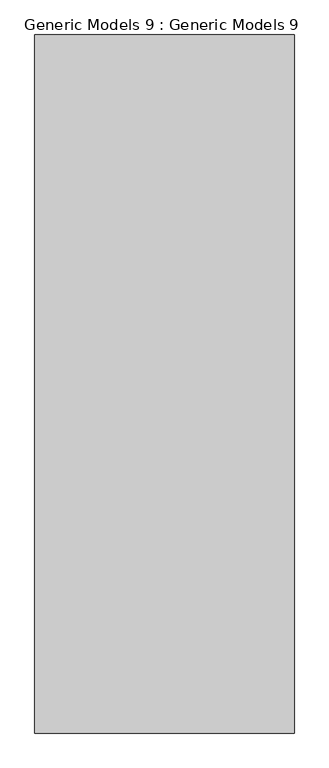
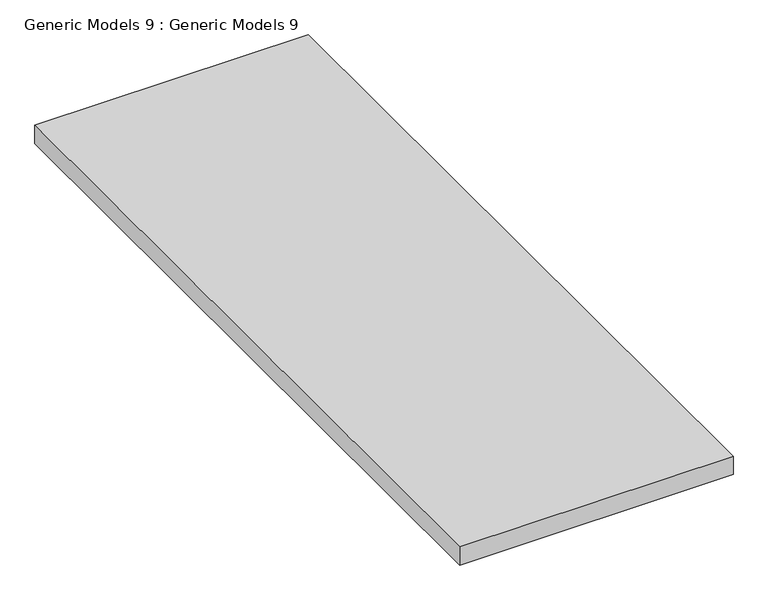
"""IFC4 building model written with IfcOpenShell, lengths in millimetres: proxy geometry, Generic Models 9 : Generic Models 9."""

from ifc_helpers import new_model, si_unit, frame, origin, place, context, project, spatial, polyline, outline, extrude, source, transform, mapped, element, save


def generic_models_9_generic_models_9_5a9dd815(model_context):
    return source(origin(), model_context, "Body", "SweptSolid", [
        extrude(outline(polyline([(-3736.8593778, -7976.2951755), (-5910.1906521, -7976.2951755), (-5910.1906521, -2131.7746485), (-3736.8593778, -2131.7746485), (-3736.8593778, -7976.2951755)])), frame((0.0, 0.0, 7010.4), z_axis=(0.0, 0.0, 1.0), x_axis=(1.0, 0.0, 0.0)), (0.0, 0.0, 1.0), 152.4),
    ])


if __name__ == "__main__":
    model = new_model("IFC4")
    model_context = context("Model", 3, world=origin())
    ifc_project = project(units=[si_unit("LENGTHUNIT", "METRE", prefix="MILLI")], contexts=[model_context])
    site = spatial("IfcSite", under=ifc_project)
    building = spatial("IfcBuilding", under=site)
    placement = place(None, origin())
    generic_models_9_generic_models_9_shape = generic_models_9_generic_models_9_5a9dd815(model_context)
    element("IfcBuildingElementProxy", 1, Name="Generic Models 9 : Generic Models 9", ObjectType="Generic Models 9 : Generic Models 9", at=placement, inside=building, context=model_context, shape_type="MappedRepresentation", body=[
        mapped(generic_models_9_generic_models_9_shape, transform((0.0, 0.0, 0.0), x_axis=(1.0, 0.0, 0.0), y_axis=(0.0, 1.0, 0.0), z_axis=(0.0, 0.0, 1.0))),
    ])
    save(model, "model.ifc")

# Revit data of these elements
# Element 1 (IfcBuildingElementProxy, "Generic Models 9 : Generic Models 9")
#   Materials on its faces: "GREY COLOUR FRAME(2)"
# Materials
#   "GREY COLOUR FRAME(2)": class "Generic", colour RGB 120 120 120, transparency 0, Cost = 0
